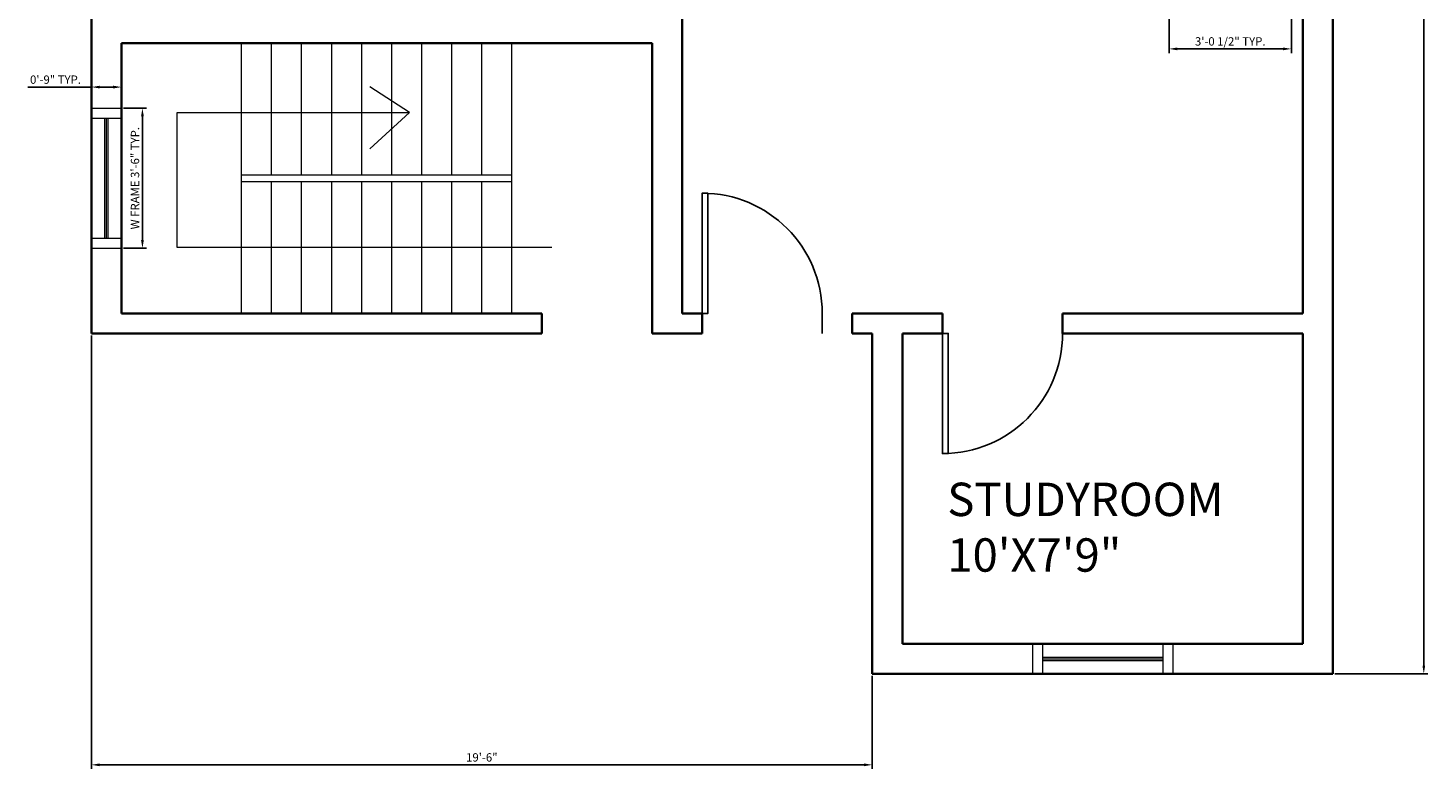
# Model space of a CAD drawing. Units: inches. Extents: x 2163 to 7246, y 928 to 2098.
# Tile 11 of 15: x 5214 to 5633, y 1429 to 1651. Entities that reach past the tile are written whole.
import ezdxf

# ---------------------------------------------------------------- set-up
doc = ezdxf.new("R2010")
doc.units = ezdxf.units.IN
for name, color, linetype, lineweight in [('A-ANNO-DIMS', 4, 'Continuous', 18), ('A-AREA-IDEN', 7, 'Continuous', 18), ('A-DOOR', 4, 'Continuous', 25), ('A-FLOR-STRS', 7, 'Continuous', 20), ('A-GLAZ', 30, 'Continuous', 20), ('A-WALL', 7, 'Continuous', 35)]:
    doc.layers.add(name, color=color, linetype=linetype, lineweight=lineweight)
doc.styles.get("Standard").update_dxf_attribs({"font": 'arial.ttf'})
doc.dimstyles.new('ISO-25', dxfattribs={"dimtxt": 2.5, "dimasz": 2.5, "dimexe": 1.25, "dimexo": 0.625, "dimtad": 1, "dimdec": 0, "dimlunit": 3, "dimtxsty": 'Standard', "dimcen": 2.5, "dimadec": 0, "dimazin": 0, "dimtfac": 1, "dimtdec": 0, "dimtmove": 0, "dimatfit": 3, "dimfxl": 1, "dimarcsym": 0})

# ---------------------------------------------------------------- blocks, each defined once
blk = doc.blocks.new('*U33')
for p, q in [((0, 0), (0, 6)), ((36, 0), (36, 6))]:
    blk.add_line(p, q)
blk.add_lwpolyline([(0, 0), (0, -36), (1.75, -36), (1.75, 0)], close=True)
blk.add_arc((0, 0), 36, 270, 0)
blk = doc.blocks.new('*U4')
for p, q in [((0, 0), (0, -6)), ((36, 0), (36, -6))]:
    blk.add_line(p, q)
blk.add_lwpolyline([(0, 0), (0, 36), (1.75, 36), (1.75, 0)], close=True)
blk.add_arc((0, 0), 36, 0, 90)
blk = doc.blocks.new('WIN-36-PLAN')
for p, q in [((0, 9), (0, 0)), ((3, 9), (3, 0)), ((39, 9), (39, 0)), ((42, 9), (42, 0)), ((3, 5), (39, 5)), ((3, 4.5), (39, 4.5)), ((3, 4), (39, 4))]:
    blk.add_line(p, q)
blk = doc.blocks.new('STAIR-DOGLEG-81')
for p, q in [((19.35, 0), (19.35, 81)), ((28.35, 41.5), (28.35, 81)), ((37.35, 41.5), (37.35, 81)), ((46.35, 41.5), (46.35, 81)), ((55.35, 41.5), (55.35, 81)), ((64.35, 41.5), (64.35, 81)), ((73.35, 41.5), (73.35, 81)), ((82.35, 41.5), (82.35, 81)), ((91.35, 41.5), (91.35, 81)), ((100.35, 0), (100.35, 81)), ((69.69, 60.16), (57.76, 67.88)), ((0, 19.75), (0, 60.16)), ((0, 60.16), (69.69, 60.16)), ((69.69, 60.16), (57.82, 49.34)), ((19.35, 41.5), (100.35, 41.5)), ((19.35, 39.5), (100.35, 39.5)), ((28.35, 0), (28.35, 39.5)), ((37.35, 0), (37.35, 39.5)), ((46.35, 0), (46.35, 39.5)), ((55.35, 0), (55.35, 39.5)), ((64.35, 0), (64.35, 39.5)), ((73.35, 0), (73.35, 39.5)), ((82.35, 0), (82.35, 39.5)), ((91.35, 0), (91.35, 39.5)), ((112.3, 19.75), (0, 19.75))]:
    blk.add_line(p, q)
blk = doc.blocks.new('*D49')
at = {"layer": 'A-ANNO-DIMS', "color": 0, "lineweight": -2, "transparency": 16777216}
for p, q in [((5242.35, 1627.46), (5249.27, 1627.46)), ((5248.02, 1587.96), (5248.02, 1624.96)), ((5242.35, 1585.46), (5249.27, 1585.46))]:
    blk.add_line(p, q, dxfattribs=at)
at = {"layer": 'A-ANNO-DIMS', "color": 0, "transparency": 16777216}
for points in [[(5247.61, 1624.96), (5248.44, 1624.96), (5248.02, 1627.46)], [(5247.61, 1587.96), (5248.44, 1587.96), (5248.02, 1585.46)]]:
    blk.add_solid(points, dxfattribs=at)
at = {"layer": 'Defpoints', "color": 0, "transparency": 16777216}
for p in [(5241.72, 1627.46), (5248.02, 1627.46), (5241.72, 1585.46)]:
    blk.add_point(p, dxfattribs=at)
at = {"layer": 'A-ANNO-DIMS', "color": 0, "transparency": 16777216, "insert": (5246.12, 1606.46), "char_height": 2.5, "attachment_point": 5, "rotation": 90}
blk.add_mtext('W FRAME 3\'-6" TYP.', dxfattribs=at)
blk = doc.blocks.new('*D50')
at = {"layer": 'A-ANNO-DIMS', "color": 0, "lineweight": -2, "transparency": 16777216}
for p, q in [((5232.72, 1633.76), (5213.73, 1633.76)), ((5232.72, 1628.08), (5232.72, 1635.01)), ((5239.22, 1633.76), (5235.22, 1633.76)), ((5241.72, 1628.08), (5241.72, 1635.01))]:
    blk.add_line(p, q, dxfattribs=at)
at = {"layer": 'A-ANNO-DIMS', "color": 0, "transparency": 16777216}
for points in [[(5235.22, 1634.17), (5235.22, 1633.34), (5232.72, 1633.76)], [(5239.22, 1634.17), (5239.22, 1633.34), (5241.72, 1633.76)]]:
    blk.add_solid(points, dxfattribs=at)
at = {"layer": 'Defpoints', "color": 0, "transparency": 16777216}
for p in [(5232.72, 1633.76), (5232.72, 1627.46), (5241.72, 1627.46)]:
    blk.add_point(p, dxfattribs=at)
at = {"layer": 'A-ANNO-DIMS', "color": 0, "transparency": 16777216, "insert": (5221.98, 1635.66), "char_height": 2.5, "attachment_point": 5}
blk.add_mtext('0\'-9" TYP.', dxfattribs=at)
blk = doc.blocks.new('*D64')
at = {"layer": 'A-ANNO-DIMS', "color": 0, "lineweight": -2, "transparency": 16777216}
for p, q in [((5555.62, 1657.18), (5555.62, 1643.95)), ((5592.29, 1657.18), (5592.29, 1643.95)), ((5558.12, 1645.2), (5589.79, 1645.2))]:
    blk.add_line(p, q, dxfattribs=at)
at = {"layer": 'A-ANNO-DIMS', "color": 0, "transparency": 16777216}
for points in [[(5558.12, 1645.62), (5558.12, 1644.78), (5555.62, 1645.2)], [(5589.79, 1645.62), (5589.79, 1644.78), (5592.29, 1645.2)]]:
    blk.add_solid(points, dxfattribs=at)
at = {"layer": 'Defpoints', "color": 0, "transparency": 16777216}
for p in [(5555.62, 1657.8), (5592.29, 1657.8), (5592.29, 1645.2)]:
    blk.add_point(p, dxfattribs=at)
at = {"layer": 'A-ANNO-DIMS', "color": 0, "transparency": 16777216, "insert": (5573.96, 1647.12), "char_height": 2.5, "attachment_point": 5}
blk.add_mtext('3\'-0 1/2" TYP.', dxfattribs=at)
blk = doc.blocks.new('*D110')
at = {"layer": 'A-ANNO-DIMS', "color": 0, "lineweight": -2, "transparency": 16777216}
for p, q in [((5605.35, 2000.96), (5633.22, 2000.96)), ((5631.97, 1998.46), (5631.97, 1460.46)), ((5605.35, 1457.96), (5633.22, 1457.96))]:
    blk.add_line(p, q, dxfattribs=at)
at = {"layer": 'A-ANNO-DIMS', "color": 0, "transparency": 16777216}
for points in [[(5631.56, 1998.46), (5632.39, 1998.46), (5631.97, 2000.96)], [(5631.56, 1460.46), (5632.39, 1460.46), (5631.97, 1457.96)]]:
    blk.add_solid(points, dxfattribs=at)
at = {"layer": 'Defpoints', "color": 0, "transparency": 16777216}
for p in [(5604.72, 2000.96), (5604.72, 1457.96), (5631.97, 1457.96)]:
    blk.add_point(p, dxfattribs=at)
at = {"layer": 'A-ANNO-DIMS', "color": 0, "transparency": 16777216, "insert": (5630.07, 1729.46), "char_height": 2.5, "attachment_point": 5, "rotation": 90}
blk.add_mtext('45\'-3"', dxfattribs=at)
blk = doc.blocks.new('*D111')
at = {"layer": 'A-ANNO-DIMS', "color": 0, "lineweight": -2, "transparency": 16777216}
for p, q in [((5232.72, 1559.33), (5232.72, 1429.46)), ((5466.72, 1457.33), (5466.72, 1429.46)), ((5235.22, 1430.71), (5464.22, 1430.71))]:
    blk.add_line(p, q, dxfattribs=at)
at = {"layer": 'A-ANNO-DIMS', "color": 0, "transparency": 16777216}
for points in [[(5235.22, 1431.12), (5235.22, 1430.29), (5232.72, 1430.71)], [(5464.22, 1431.12), (5464.22, 1430.29), (5466.72, 1430.71)]]:
    blk.add_solid(points, dxfattribs=at)
at = {"layer": 'Defpoints', "color": 0, "transparency": 16777216}
for p in [(5232.72, 1559.96), (5466.72, 1457.96), (5466.72, 1430.71)]:
    blk.add_point(p, dxfattribs=at)
at = {"layer": 'A-ANNO-DIMS', "color": 0, "transparency": 16777216, "insert": (5349.72, 1432.61), "char_height": 2.5, "attachment_point": 5}
blk.add_mtext('19\'-6"', dxfattribs=at)

msp = doc.modelspace()

# ---------------------------------------------------------------- linework, layer by layer
at = {"layer": 'A-WALL'}
for p, q in [((5232.72, 1559.96), (5232.72, 2000.96)), ((5604.72, 2000.96), (5604.72, 1457.96)), ((5595.72, 1841.96), (5595.72, 1565.96)), ((5409.72, 1781.96), (5409.72, 1565.96)), ((5241.72, 1646.96), (5400.72, 1646.96)), ((5241.72, 1565.96), (5241.72, 1646.96)), ((5400.72, 1646.96), (5400.72, 1559.96)), ((5241.72, 1565.96), (5367.72, 1565.96)), ((5367.72, 1559.96), (5367.72, 1565.96)), ((5409.72, 1565.96), (5415.72, 1565.96)), ((5415.72, 1565.96), (5415.72, 1559.96)), ((5460.72, 1565.96), (5460.72, 1559.96)), ((5460.72, 1565.96), (5487.72, 1565.96)), ((5487.72, 1565.96), (5487.72, 1559.96)), ((5523.72, 1565.96), (5523.72, 1559.96)), ((5523.72, 1565.96), (5595.72, 1565.96)), ((5232.72, 1559.96), (5367.72, 1559.96)), ((5400.72, 1559.96), (5415.72, 1559.96)), ((5460.72, 1559.96), (5466.72, 1559.96)), ((5466.72, 1559.96), (5466.72, 1457.96)), ((5475.72, 1559.96), (5475.72, 1466.96)), ((5475.72, 1559.96), (5487.72, 1559.96)), ((5523.72, 1559.96), (5595.72, 1559.96)), ((5595.72, 1559.96), (5595.72, 1466.96)), ((5595.72, 1466.96), (5475.72, 1466.96)), ((5604.72, 1457.96), (5466.72, 1457.96))]:
    msp.add_line(p, q, dxfattribs=at)

# ---------------------------------------------------------------- block references
at = {"layer": 'A-DOOR'}
for name, p in [('*U4', (5415.72, 1565.96)), ('*U33', (5487.72, 1559.96))]:
    msp.add_blockref(name, p, dxfattribs=at)
at = {"layer": 'A-FLOR-STRS'}
msp.add_blockref('STAIR-DOGLEG-81', (5258.38, 1565.96), dxfattribs=at)
at = {"layer": 'A-GLAZ', "rotation": 90}
msp.add_blockref('WIN-36-PLAN', (5241.72, 1585.46), dxfattribs=at)
at = {"layer": 'A-GLAZ'}
msp.add_blockref('WIN-36-PLAN', (5514.72, 1457.96), dxfattribs=at)

# ---------------------------------------------------------------- texts
at = {"layer": 'A-AREA-IDEN', "insert": (5489.18, 1515.24), "char_height": 10, "attachment_point": 1}
msp.add_mtext_dynamic_manual_height_columns('STUDYROOM\\P10\'X7\'9"', width=90.7352, gutter_width=12.5, heights=[0], dxfattribs=at)

# ---------------------------------------------------------------- dimensions: what is measured, and where the dimension line sits
at = {"layer": 'A-ANNO-DIMS'}
dim = msp.add_linear_dim(base=(5631.97, 1457.96), p1=(5604.72, 2000.96), p2=(5604.72, 1457.96), angle=90, dimstyle='ISO-25', override={"dimdec": 1, "dimlfac": 1, "dimrnd": 0, "dimzin": 1, "dimdsep": 46, "dimlunit": 4, "dimfrac": 2}, dxfattribs=at)
dim.commit()
dim.dimension.update_dxf_attribs({"geometry": '*D110', "text_midpoint": (5630.07, 1729.46)})
dim = msp.add_linear_dim(base=(5592.29, 1645.2), p1=(5555.62, 1657.8), p2=(5592.29, 1657.8), text='<> TYP.', dimstyle='ISO-25', override={"dimdec": 1, "dimlfac": 1, "dimrnd": 0, "dimzin": 1, "dimdsep": 46, "dimlunit": 4, "dimfrac": 2}, dxfattribs=at)
dim.commit()
dim.dimension.update_dxf_attribs({"geometry": '*D64', "text_midpoint": (5573.96, 1647.12)})
for base, p1, p2, angle, text, picture, middle in [((5232.72, 1633.76), (5241.72, 1627.46), (5232.72, 1627.46), 180, '<> TYP.', '*D50', (5221.98, 1635.66)), ((5248.02, 1627.46), (5241.72, 1585.46), (5241.72, 1627.46), 90, 'W FRAME <> TYP.', '*D49', (5246.12, 1606.46))]:
    dim = msp.add_linear_dim(base=base, p1=p1, p2=p2, angle=angle, text=text, dimstyle='ISO-25', override={"dimdec": 1, "dimlfac": 1, "dimrnd": 0, "dimzin": 1, "dimdsep": 46, "dimlunit": 4, "dimfrac": 2}, dxfattribs=at)
    dim.commit()
    dim.dimension.update_dxf_attribs({"geometry": picture, "text_midpoint": middle})
dim = msp.add_linear_dim(base=(5466.72, 1430.71), p1=(5232.72, 1559.96), p2=(5466.72, 1457.96), dimstyle='ISO-25', override={"dimdec": 1, "dimlfac": 1, "dimrnd": 0, "dimzin": 1, "dimdsep": 46, "dimlunit": 4, "dimfrac": 2}, dxfattribs=at)
dim.commit()
dim.dimension.update_dxf_attribs({"geometry": '*D111', "text_midpoint": (5349.72, 1432.61)})

doc.saveas('drawing.dxf')
